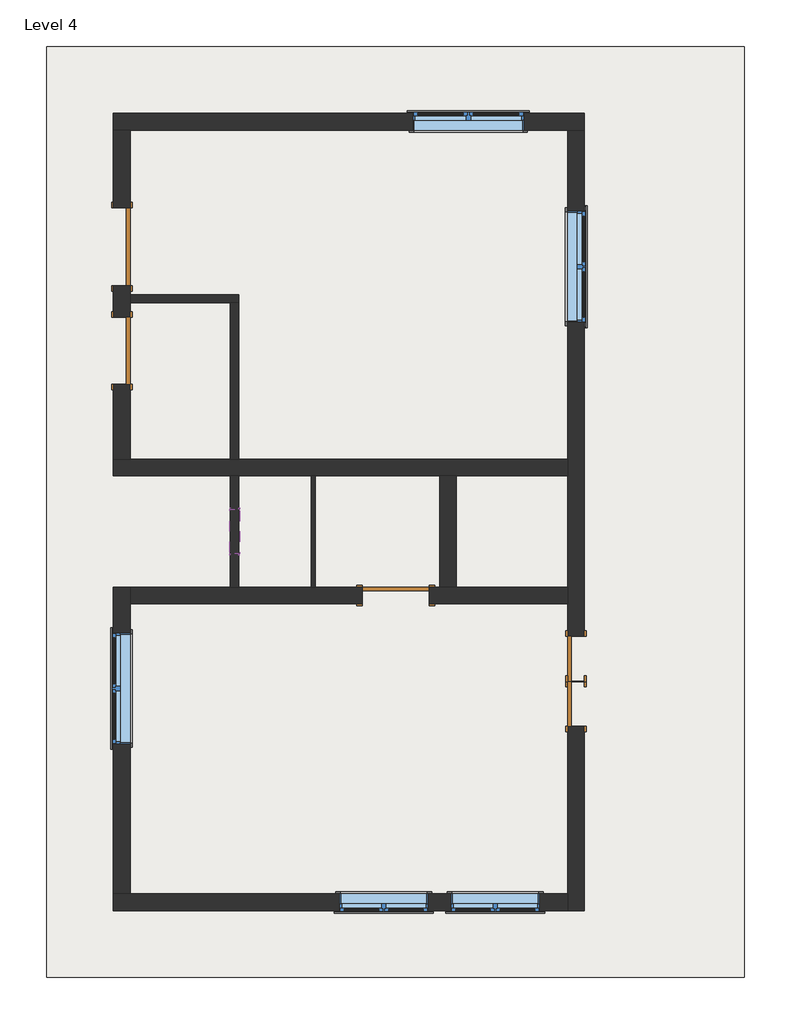
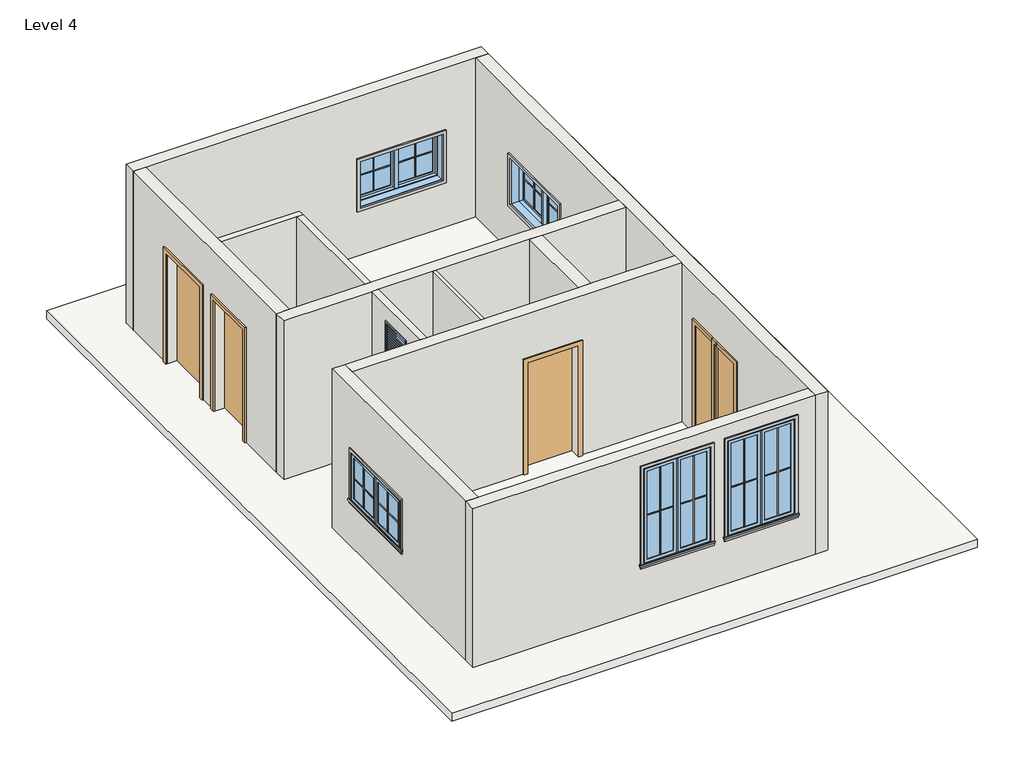
# One storey, incomplete: 20 proxies, 12 walls, 6 windows, 5 doors, 1 roof.
"""IFC4 building model written with IfcOpenShell, lengths in millimetres."""

from ifc_helpers import new_model, si_unit, frame, origin, place, context, project, spatial, polyline, outline, extrude, faceted_brep, transform, mapped, element, save
from components import muntin_pattern_2x2_muntin_pattern_2x2_9352d081, muntin_pattern_2x2_muntin_pattern_2x2_5c2cbe28, muntin_pattern_2x2_muntin_pattern_2x2_2b4d9f72, muntin_pattern_2x2_muntin_pattern_2x2_ef995ed3, trim_window_exterior_flat_with_sill_979bde60, trim_window_exterior_flat_with_sill_b7e4d11c, trim_window_interior_flat_picture_frame_7883d11b, trim_window_interior_flat_picture_frame_936b8d2a, single_flush_door_2_0d3b4037, single_flush_door_2_4a3212df, door_a90ba1ad, door_0ca8825f, door_9d399b00, window_casement_double_c1d95f0f, window_casement_double_wall_4_6ca1769e, window_d39e7ecb

model = new_model("IFC4")

# Units and contexts
model_context = context("Model", 3, world=origin())
ifc_project = project(units=[si_unit("LENGTHUNIT", "METRE", prefix="MILLI")], contexts=[model_context])

# Site, building, storey
site = spatial("IfcSite", under=ifc_project)
building = spatial("IfcBuilding", under=site)
storey = spatial("IfcBuildingStorey", under=building, Name="Level 4", Elevation=6400.8)

# Proxies
placement = place(None, origin())
muntin_pattern_2x2_muntin_pattern_2x2_shape = muntin_pattern_2x2_muntin_pattern_2x2_9352d081(model_context)
element("IfcBuildingElementProxy", 1, Name="Muntin Pattern_2x2 : Muntin Pattern_2x2", ObjectType="Muntin Pattern_2x2 : Muntin Pattern_2x2", at=placement, inside=storey, context=model_context, shape_type="MappedRepresentation", body=[
    mapped(muntin_pattern_2x2_muntin_pattern_2x2_shape, transform((-4785.3510342, -2707.8617544, 7385.05), x_axis=(0.0, 1.0, 0.0), y_axis=(-1.0, 0.0, 0.0), z_axis=(0.0, 0.0, 1.0))),
])
element("IfcBuildingElementProxy", 2, Name="Muntin Pattern_2x2 : Muntin Pattern_2x2", ObjectType="Muntin Pattern_2x2 : Muntin Pattern_2x2", at=placement, inside=storey, context=model_context, shape_type="MappedRepresentation", body=[
    mapped(muntin_pattern_2x2_muntin_pattern_2x2_shape, transform((1634.4989658, 3816.7632456, 7385.05), x_axis=(0.0, -1.0, 0.0), y_axis=(1.0, 0.0, 0.0), z_axis=(0.0, 0.0, 1.0))),
])
element("IfcBuildingElementProxy", 3, Name="Muntin Pattern_2x2 : Muntin Pattern_2x2", ObjectType="Muntin Pattern_2x2 : Muntin Pattern_2x2", at=placement, inside=storey, context=model_context, shape_type="MappedRepresentation", body=[
    mapped(muntin_pattern_2x2_muntin_pattern_2x2_shape, transform((-322.8885342, 5523.3257456, 7385.05), x_axis=(1.0, 0.0, 0.0), y_axis=(0.0, 1.0, 0.0), z_axis=(0.0, 0.0, 1.0))),
])
muntin_pattern_2x2_muntin_pattern_2x2_2_shape = muntin_pattern_2x2_muntin_pattern_2x2_5c2cbe28(model_context)
element("IfcBuildingElementProxy", 4, Name="Muntin Pattern_2x2 : Muntin Pattern_2x2", ObjectType="Muntin Pattern_2x2 : Muntin Pattern_2x2", at=placement, inside=storey, context=model_context, shape_type="MappedRepresentation", body=[
    mapped(muntin_pattern_2x2_muntin_pattern_2x2_2_shape, transform((-4785.3510342, -1949.0367544, 7385.05), x_axis=(0.0, -1.0, 0.0), y_axis=(1.0, 0.0, 0.0), z_axis=(0.0, 0.0, 1.0))),
])
element("IfcBuildingElementProxy", 5, Name="Muntin Pattern_2x2 : Muntin Pattern_2x2", ObjectType="Muntin Pattern_2x2 : Muntin Pattern_2x2", at=placement, inside=storey, context=model_context, shape_type="MappedRepresentation", body=[
    mapped(muntin_pattern_2x2_muntin_pattern_2x2_2_shape, transform((1634.4989658, 3057.9382456, 7385.05), x_axis=(0.0, 1.0, 0.0), y_axis=(-1.0, 0.0, 0.0), z_axis=(0.0, 0.0, 1.0))),
])
element("IfcBuildingElementProxy", 6, Name="Muntin Pattern_2x2 : Muntin Pattern_2x2", ObjectType="Muntin Pattern_2x2 : Muntin Pattern_2x2", at=placement, inside=storey, context=model_context, shape_type="MappedRepresentation", body=[
    mapped(muntin_pattern_2x2_muntin_pattern_2x2_2_shape, transform((435.9364658, 5523.3257456, 7385.05), x_axis=(-1.0, 0.0, 0.0), y_axis=(0.0, -1.0, 0.0), z_axis=(0.0, 0.0, 1.0))),
])
muntin_pattern_2x2_muntin_pattern_2x2_3_shape = muntin_pattern_2x2_muntin_pattern_2x2_2b4d9f72(model_context)
element("IfcBuildingElementProxy", 7, Name="Muntin Pattern_2x2 : Muntin Pattern_2x2", ObjectType="Muntin Pattern_2x2 : Muntin Pattern_2x2", at=placement, inside=storey, context=model_context, shape_type="MappedRepresentation", body=[
    mapped(muntin_pattern_2x2_muntin_pattern_2x2_3_shape, transform((-795.9635342, -5354.2242544, 7385.05), x_axis=(-1.0, 0.0, 0.0), y_axis=(0.0, -1.0, 0.0), z_axis=(0.0, 0.0, 1.0))),
])
element("IfcBuildingElementProxy", 8, Name="Muntin Pattern_2x2 : Muntin Pattern_2x2", ObjectType="Muntin Pattern_2x2 : Muntin Pattern_2x2", at=placement, inside=storey, context=model_context, shape_type="MappedRepresentation", body=[
    mapped(muntin_pattern_2x2_muntin_pattern_2x2_3_shape, transform((728.0364658, -5354.2242544, 7385.05), x_axis=(-1.0, 0.0, 0.0), y_axis=(0.0, -1.0, 0.0), z_axis=(0.0, 0.0, 1.0))),
])
muntin_pattern_2x2_muntin_pattern_2x2_4_shape = muntin_pattern_2x2_muntin_pattern_2x2_ef995ed3(model_context)
element("IfcBuildingElementProxy", 9, Name="Muntin Pattern_2x2 : Muntin Pattern_2x2", ObjectType="Muntin Pattern_2x2 : Muntin Pattern_2x2", at=placement, inside=storey, context=model_context, shape_type="MappedRepresentation", body=[
    mapped(muntin_pattern_2x2_muntin_pattern_2x2_4_shape, transform((-1402.3885342, -5354.2242544, 7385.05), x_axis=(1.0, 0.0, 0.0), y_axis=(0.0, 1.0, 0.0), z_axis=(0.0, 0.0, 1.0))),
])
element("IfcBuildingElementProxy", 10, Name="Muntin Pattern_2x2 : Muntin Pattern_2x2", ObjectType="Muntin Pattern_2x2 : Muntin Pattern_2x2", at=placement, inside=storey, context=model_context, shape_type="MappedRepresentation", body=[
    mapped(muntin_pattern_2x2_muntin_pattern_2x2_4_shape, transform((121.6114658, -5354.2242544, 7385.05), x_axis=(1.0, 0.0, 0.0), y_axis=(0.0, 1.0, 0.0), z_axis=(0.0, 0.0, 1.0))),
])
trim_window_exterior_flat_with_sill_shape = trim_window_exterior_flat_with_sill_979bde60(model_context)
element("IfcBuildingElementProxy", 11, Name="Trim-Window-Exterior-Flat : with Sill", ObjectType="Trim-Window-Exterior-Flat : with Sill", at=placement, inside=storey, context=model_context, shape_type="MappedRepresentation", body=[
    mapped(trim_window_exterior_flat_with_sill_shape, transform((-4794.8760342, -2328.4492544, 8229.6), x_axis=(0.0, -1.0, 0.0), y_axis=(0.0, 0.0, 1.0), z_axis=(-1.0, 0.0, 0.0))),
])
element("IfcBuildingElementProxy", 12, Name="Trim-Window-Exterior-Flat : with Sill", ObjectType="Trim-Window-Exterior-Flat : with Sill", at=placement, inside=storey, context=model_context, shape_type="MappedRepresentation", body=[
    mapped(trim_window_exterior_flat_with_sill_shape, transform((1644.0239658, 3437.3507456, 8229.6), x_axis=(0.0, 1.0, 0.0), y_axis=(0.0, 0.0, 1.0), z_axis=(1.0, 0.0, 0.0))),
])
element("IfcBuildingElementProxy", 13, Name="Trim-Window-Exterior-Flat : with Sill", ObjectType="Trim-Window-Exterior-Flat : with Sill", at=placement, inside=storey, context=model_context, shape_type="MappedRepresentation", body=[
    mapped(trim_window_exterior_flat_with_sill_shape, transform((56.5239658, 5532.8507456, 8229.6), x_axis=(-1.0, 0.0, 0.0), y_axis=(0.0, 0.0, 1.0), z_axis=(0.0, 1.0, 0.0))),
])
trim_window_exterior_flat_with_sill_2_shape = trim_window_exterior_flat_with_sill_b7e4d11c(model_context)
element("IfcBuildingElementProxy", 14, Name="Trim-Window-Exterior-Flat : with Sill", ObjectType="Trim-Window-Exterior-Flat : with Sill", at=placement, inside=storey, context=model_context, shape_type="MappedRepresentation", body=[
    mapped(trim_window_exterior_flat_with_sill_2_shape, transform((-1099.1760342, -5363.7492544, 9144.0), x_axis=(1.0, 0.0, 0.0), y_axis=(0.0, 0.0, 1.0), z_axis=(0.0, -1.0, 0.0))),
])
element("IfcBuildingElementProxy", 15, Name="Trim-Window-Exterior-Flat : with Sill", ObjectType="Trim-Window-Exterior-Flat : with Sill", at=placement, inside=storey, context=model_context, shape_type="MappedRepresentation", body=[
    mapped(trim_window_exterior_flat_with_sill_2_shape, transform((424.8239658, -5363.7492544, 9144.0), x_axis=(1.0, 0.0, 0.0), y_axis=(0.0, 0.0, 1.0), z_axis=(0.0, -1.0, 0.0))),
])
trim_window_interior_flat_picture_frame_shape = trim_window_interior_flat_picture_frame_7883d11b(model_context)
element("IfcBuildingElementProxy", 16, Name="Trim-Window-Interior-Flat : Picture Frame", ObjectType="Trim-Window-Interior-Flat : Picture Frame", at=placement, inside=storey, context=model_context, shape_type="MappedRepresentation", body=[
    mapped(trim_window_interior_flat_picture_frame_shape, transform((-4566.2760342, -2328.4492544, 8229.6), x_axis=(0.0, 1.0, 0.0), y_axis=(0.0, 0.0, 1.0), z_axis=(1.0, 0.0, 0.0))),
])
element("IfcBuildingElementProxy", 17, Name="Trim-Window-Interior-Flat : Picture Frame", ObjectType="Trim-Window-Interior-Flat : Picture Frame", at=placement, inside=storey, context=model_context, shape_type="MappedRepresentation", body=[
    mapped(trim_window_interior_flat_picture_frame_shape, transform((1415.4239658, 3437.3507456, 8229.6), x_axis=(0.0, -1.0, 0.0), y_axis=(0.0, 0.0, 1.0), z_axis=(-1.0, 0.0, 0.0))),
])
element("IfcBuildingElementProxy", 18, Name="Trim-Window-Interior-Flat : Picture Frame", ObjectType="Trim-Window-Interior-Flat : Picture Frame", at=placement, inside=storey, context=model_context, shape_type="MappedRepresentation", body=[
    mapped(trim_window_interior_flat_picture_frame_shape, transform((56.5239658, 5304.2507456, 8229.6), x_axis=(1.0, 0.0, 0.0), y_axis=(0.0, 0.0, 1.0), z_axis=(0.0, -1.0, 0.0))),
])
trim_window_interior_flat_picture_frame_2_shape = trim_window_interior_flat_picture_frame_936b8d2a(model_context)
element("IfcBuildingElementProxy", 19, Name="Trim-Window-Interior-Flat : Picture Frame", ObjectType="Trim-Window-Interior-Flat : Picture Frame", at=placement, inside=storey, context=model_context, shape_type="MappedRepresentation", body=[
    mapped(trim_window_interior_flat_picture_frame_2_shape, transform((-1099.1760342, -5135.1492544, 9144.0), x_axis=(-1.0, 0.0, 0.0), y_axis=(0.0, 0.0, 1.0), z_axis=(0.0, 1.0, 0.0))),
])
element("IfcBuildingElementProxy", 20, Name="Trim-Window-Interior-Flat : Picture Frame", ObjectType="Trim-Window-Interior-Flat : Picture Frame", at=placement, inside=storey, context=model_context, shape_type="MappedRepresentation", body=[
    mapped(trim_window_interior_flat_picture_frame_2_shape, transform((424.8239658, -5135.1492544, 9144.0), x_axis=(-1.0, 0.0, 0.0), y_axis=(0.0, 0.0, 1.0), z_axis=(0.0, 1.0, 0.0))),
])

# Doors
single_flush_door_2_shape = single_flush_door_2_0d3b4037(model_context)
element("IfcDoor", 21, ObjectType="Single-Flush : door 2'", at=placement, inside=storey, context=model_context, shape_type="MappedRepresentation", body=[
    mapped(single_flush_door_2_shape, transform((1529.7239658, -1922.0492544, 6400.8), x_axis=(0.0, 1.0, 0.0), y_axis=(-1.0, 0.0, 0.0), z_axis=(0.0, 0.0, 1.0))),
])
single_flush_door_2_2_shape = single_flush_door_2_4a3212df(model_context)
element("IfcDoor", 22, ObjectType="Single-Flush : door 2'", at=placement, inside=storey, context=model_context, shape_type="MappedRepresentation", body=[
    mapped(single_flush_door_2_2_shape, transform((1529.7239658, -2537.9992544, 6400.8), x_axis=(0.0, -1.0, 0.0), y_axis=(1.0, 0.0, 0.0), z_axis=(0.0, 0.0, 1.0))),
])
door_shape = door_a90ba1ad(model_context)
element("IfcDoor", 23, ObjectType="Single-Flush : door 2'6\"", at=placement, inside=storey, context=model_context, shape_type="MappedRepresentation", body=[
    mapped(door_shape, transform((-4680.5760342, 2288.0007456, 6400.8), x_axis=(0.0, 1.0, 0.0), y_axis=(-1.0, 0.0, 0.0), z_axis=(0.0, 0.0, 1.0))),
])
door_2_shape = door_0ca8825f(model_context)
element("IfcDoor", 24, ObjectType="Single-Flush : door 2'6\"", at=placement, inside=storey, context=model_context, shape_type="MappedRepresentation", body=[
    mapped(door_2_shape, transform((-934.0760342, -1058.4492544, 6400.8), x_axis=(1.0, 0.0, 0.0), y_axis=(0.0, 1.0, 0.0), z_axis=(0.0, 0.0, 1.0))),
])
door_3_shape = door_9d399b00(model_context)
element("IfcDoor", 25, ObjectType="Single-Flush : door 3'6\"", at=placement, inside=storey, context=model_context, shape_type="MappedRepresentation", body=[
    mapped(door_3_shape, transform((-4680.5760342, 3710.4007456, 6400.8), x_axis=(0.0, -1.0, 0.0), y_axis=(1.0, 0.0, 0.0), z_axis=(0.0, 0.0, 1.0))),
])

# Roof
element("IfcRoof", 26, ObjectType="roof 6\"", at=placement, inside=storey, context=model_context, shape_type="SweptSolid", body=[
    extrude(outline(polyline([(-5709.2760342, 6447.2507456), (3828.4239658, 6447.2507456), (3828.4239658, -6278.1492544), (-5709.2760342, -6278.1492544), (-5709.2760342, 6447.2507456)])), frame((0.0, 0.0, 6248.4), z_axis=(0.0, 0.0, 1.0), x_axis=(1.0, 0.0, 0.0)), (0.0, 0.0, 1.0), 152.4),
])

# Walls
element("IfcWall", 27, ObjectType="wall 2\"", at=placement, inside=storey, context=model_context, shape_type="SweptSolid", body=[
    extrude(outline(polyline([(-2089.7760342, -944.1492544), (-2089.7760342, 579.8507456), (-2038.9760342, 579.8507456), (-2038.9760342, -944.1492544), (-2089.7760342, -944.1492544)])), frame((0.0, 0.0, 6400.8), z_axis=(0.0, 0.0, 1.0), x_axis=(1.0, 0.0, 0.0)), (0.0, 0.0, 1.0), 3048.0),
])
element("IfcWall", 28, ObjectType="wall 4.5\"", at=placement, inside=storey, context=model_context, shape_type="Brep", body=[
    faceted_brep([(-4566.2760342, 2942.0507456, 6400.8), (-3194.6760342, 2942.0507456, 6400.8), (-3080.3760342, 2942.0507456, 6400.8), (-3080.3760342, 2942.0507456, 9448.8), (-3194.6760342, 2942.0507456, 9448.8), (-4566.2760342, 2942.0507456, 9448.8), (-4566.2760342, 3056.3507456, 6400.8), (-4566.2760342, 3056.3507456, 9448.8), (-3080.3760342, 3056.3507456, 9448.8), (-3080.3760342, 3056.3507456, 6400.8)], [[[0, 1, 2, 3, 4, 5]], [[6, 7, 8, 9]], [[2, 1, 0, 6, 9]], [[0, 5, 7, 6]], [[3, 2, 9, 8]], [[5, 4, 3, 8, 7]]]),
])
element("IfcWall", 29, ObjectType="wall 4.5\"", at=placement, inside=storey, context=model_context, shape_type="SweptSolid", body=[
    extrude(outline(polyline([(-3194.6760342, 808.4507456), (-3194.6760342, 2942.0507456), (-3080.3760342, 2942.0507456), (-3080.3760342, 808.4507456), (-3194.6760342, 808.4507456)])), frame((0.0, 0.0, 6400.8), z_axis=(0.0, 0.0, 1.0), x_axis=(1.0, 0.0, 0.0)), (0.0, 0.0, 1.0), 3048.0),
])
element("IfcWall", 30, ObjectType="wall 4.5\"", at=placement, inside=storey, context=model_context, shape_type="SweptSolid", body=[
    extrude(outline(polyline([(579.8507456, 6400.8), (-944.1492544, 6400.8), (-944.1492544, 9448.8), (579.8507456, 9448.8), (579.8507456, 6400.8)]), holes=[polyline([(-486.9492544, 9144.0), (-486.9492544, 8534.4), (122.6507456, 8534.4), (122.6507456, 9144.0), (-486.9492544, 9144.0)])]), frame((-3194.6760342, 0.0, 0.0), z_axis=(1.0, 0.0, 0.0), x_axis=(0.0, 1.0, 0.0)), (0.0, 0.0, 1.0), 114.3),
])
element("IfcWall", 31, ObjectType="wall 9\"", at=placement, inside=storey, context=model_context, shape_type="Brep", body=[
    faceted_brep([(-4794.8760342, 5304.2507456, 6400.8), (-4566.2760342, 5304.2507456, 6400.8), (1415.4239658, 5304.2507456, 6400.8), (1644.0239658, 5304.2507456, 6400.8), (1644.0239658, 5304.2507456, 9448.8), (1415.4239658, 5304.2507456, 9448.8), (-4566.2760342, 5304.2507456, 9448.8), (-4794.8760342, 5304.2507456, 9448.8), (818.5239658, 5304.2507456, 8229.6), (818.5239658, 5304.2507456, 7315.2), (-705.4760342, 5304.2507456, 7315.2), (-705.4760342, 5304.2507456, 8229.6), (-4794.8760342, 5532.8507456, 6400.8), (-4794.8760342, 5532.8507456, 9448.8), (1644.0239658, 5532.8507456, 9448.8), (1644.0239658, 5532.8507456, 6400.8), (818.5239658, 5532.8507456, 8229.6), (-705.4760342, 5532.8507456, 8229.6), (-705.4760342, 5532.8507456, 7315.2), (818.5239658, 5532.8507456, 7315.2)], [[[0, 1, 2, 3, 4, 5, 6, 7], [8, 9, 10, 11]], [[12, 13, 14, 15], [16, 17, 18, 19]], [[3, 2, 1, 0, 12, 15]], [[4, 3, 15, 14]], [[0, 7, 13, 12]], [[9, 8, 16, 19]], [[10, 9, 19, 18]], [[11, 10, 18, 17]], [[8, 11, 17, 16]], [[7, 6, 5, 4, 14, 13]]]),
])
element("IfcWall", 32, ObjectType="wall 9\"", at=placement, inside=storey, context=model_context, shape_type="Brep", body=[
    faceted_brep([(1415.4239658, 5304.2507456, 9448.8), (1415.4239658, 5304.2507456, 6400.8), (1415.4239658, 808.4507456, 6400.8), (1415.4239658, 579.8507456, 6400.8), (1415.4239658, -944.1492544, 6400.8), (1415.4239658, -1172.7492544, 6400.8), (1415.4239658, -1617.2492544, 6400.8), (1415.4239658, -1617.2492544, 8534.4), (1415.4239658, -2226.8492544, 8534.4), (1415.4239658, -2226.8492544, 6400.8), (1415.4239658, -2233.1992544, 6400.8), (1415.4239658, -2233.1992544, 8534.4), (1415.4239658, -2842.7992544, 8534.4), (1415.4239658, -2842.7992544, 6400.8), (1415.4239658, -5135.1492544, 6400.8), (1415.4239658, -5363.7492544, 6400.8), (1415.4239658, -5363.7492544, 9448.8), (1415.4239658, -5135.1492544, 9448.8), (1415.4239658, -1172.7492544, 9448.8), (1415.4239658, -944.1492544, 9448.8), (1415.4239658, 579.8507456, 9448.8), (1415.4239658, 808.4507456, 9448.8), (1415.4239658, 2675.3507456, 8229.6), (1415.4239658, 2675.3507456, 7315.2), (1415.4239658, 4199.3507456, 7315.2), (1415.4239658, 4199.3507456, 8229.6), (1644.0239658, 5304.2507456, 6400.8), (1644.0239658, 5304.2507456, 9448.8), (1644.0239658, -5363.7492544, 9448.8), (1644.0239658, -5363.7492544, 6400.8), (1644.0239658, -2842.7992544, 6400.8), (1644.0239658, -2842.7992544, 8534.4), (1644.0239658, -2233.1992544, 8534.4), (1644.0239658, -2233.1992544, 6400.8), (1644.0239658, -2226.8492544, 6400.8), (1644.0239658, -2226.8492544, 8534.4), (1644.0239658, -1617.2492544, 8534.4), (1644.0239658, -1617.2492544, 6400.8), (1644.0239658, 2675.3507456, 8229.6), (1644.0239658, 4199.3507456, 8229.6), (1644.0239658, 4199.3507456, 7315.2), (1644.0239658, 2675.3507456, 7315.2)], [[[0, 1, 2, 3, 4, 5, 6, 7, 8, 9, 10, 11, 12, 13, 14, 15, 16, 17, 18, 19, 20, 21], [22, 23, 24, 25]], [[26, 27, 28, 29, 30, 31, 32, 33, 34, 35, 36, 37], [38, 39, 40, 41]], [[1, 26, 37, 6, 5, 4, 3, 2]], [[29, 15, 14, 13, 30]], [[9, 34, 33, 10]], [[1, 0, 27, 26]], [[16, 15, 29, 28]], [[23, 22, 38, 41]], [[24, 23, 41, 40]], [[25, 24, 40, 39]], [[22, 25, 39, 38]], [[7, 6, 37, 36]], [[8, 7, 36, 35]], [[9, 8, 35, 34]], [[12, 31, 30, 13]], [[31, 12, 11, 32]], [[32, 11, 10, 33]], [[0, 21, 20, 19, 18, 17, 16, 28, 27]]]),
])
element("IfcWall", 33, ObjectType="wall 9\"", at=placement, inside=storey, context=model_context, shape_type="Brep", body=[
    faceted_brep([(1415.4239658, 808.4507456, 6400.8), (-3080.3760342, 808.4507456, 6400.8), (-3194.6760342, 808.4507456, 6400.8), (-4566.2760342, 808.4507456, 6400.8), (-4794.8760342, 808.4507456, 6400.8), (-4794.8760342, 808.4507456, 9448.8), (-4566.2760342, 808.4507456, 9448.8), (-3194.6760342, 808.4507456, 9448.8), (-3080.3760342, 808.4507456, 9448.8), (1415.4239658, 808.4507456, 9448.8), (1415.4239658, 579.8507456, 6400.8), (1415.4239658, 579.8507456, 9448.8), (-108.5760342, 579.8507456, 9448.8), (-337.1760342, 579.8507456, 9448.8), (-2038.9760342, 579.8507456, 9448.8), (-2089.7760342, 579.8507456, 9448.8), (-3080.3760342, 579.8507456, 9448.8), (-3194.6760342, 579.8507456, 9448.8), (-4794.8760342, 579.8507456, 9448.8), (-4794.8760342, 579.8507456, 6400.8), (-3194.6760342, 579.8507456, 6400.8), (-3080.3760342, 579.8507456, 6400.8), (-2089.7760342, 579.8507456, 6400.8), (-2038.9760342, 579.8507456, 6400.8), (-337.1760342, 579.8507456, 6400.8), (-108.5760342, 579.8507456, 6400.8)], [[[0, 1, 2, 3, 4, 5, 6, 7, 8, 9]], [[10, 11, 12, 13, 14, 15, 16, 17, 18, 19, 20, 21, 22, 23, 24, 25]], [[4, 3, 2, 1, 0, 10, 25, 24, 23, 22, 21, 20, 19]], [[0, 9, 11, 10]], [[5, 4, 19, 18]], [[9, 8, 7, 6, 5, 18, 17, 16, 15, 14, 13, 12, 11]]]),
])
element("IfcWall", 34, ObjectType="wall 9\"", at=placement, inside=storey, context=model_context, shape_type="Brep", body=[
    faceted_brep([(-4566.2760342, 2745.2007456, 8534.4), (-4566.2760342, 2745.2007456, 6400.8), (-4566.2760342, 2942.0507456, 6400.8), (-4566.2760342, 3056.3507456, 6400.8), (-4566.2760342, 3177.0007456, 6400.8), (-4566.2760342, 3177.0007456, 8534.4), (-4566.2760342, 4243.8007456, 8534.4), (-4566.2760342, 4243.8007456, 6400.8), (-4566.2760342, 5304.2507456, 6400.8), (-4566.2760342, 5304.2507456, 9448.8), (-4566.2760342, 3056.3507456, 9448.8), (-4566.2760342, 2942.0507456, 9448.8), (-4566.2760342, 808.4507456, 9448.8), (-4566.2760342, 808.4507456, 6400.8), (-4566.2760342, 1830.8007456, 6400.8), (-4566.2760342, 1830.8007456, 8534.4), (-4794.8760342, 3177.0007456, 6400.8), (-4794.8760342, 2745.2007456, 6400.8), (-4794.8760342, 2745.2007456, 8534.4), (-4794.8760342, 1830.8007456, 8534.4), (-4794.8760342, 1830.8007456, 6400.8), (-4794.8760342, 808.4507456, 6400.8), (-4794.8760342, 808.4507456, 9448.8), (-4794.8760342, 5304.2507456, 9448.8), (-4794.8760342, 5304.2507456, 6400.8), (-4794.8760342, 4243.8007456, 6400.8), (-4794.8760342, 4243.8007456, 8534.4), (-4794.8760342, 3177.0007456, 8534.4)], [[[0, 1, 2, 3, 4, 5, 6, 7, 8, 9, 10, 11, 12, 13, 14, 15]], [[16, 17, 18, 19, 20, 21, 22, 23, 24, 25, 26, 27]], [[25, 24, 8, 7]], [[14, 13, 21, 20]], [[4, 3, 2, 1, 17, 16]], [[9, 8, 24, 23]], [[13, 12, 22, 21]], [[5, 4, 16, 27]], [[6, 5, 27, 26]], [[7, 6, 26, 25]], [[18, 17, 1, 0]], [[19, 18, 0, 15]], [[20, 19, 15, 14]], [[12, 11, 10, 9, 23, 22]]]),
])
element("IfcWall", 35, ObjectType="wall 9\"", at=placement, inside=storey, context=model_context, shape_type="Brep", body=[
    faceted_brep([(1415.4239658, -5135.1492544, 6400.8), (-4566.2760342, -5135.1492544, 6400.8), (-4794.8760342, -5135.1492544, 6400.8), (-4794.8760342, -5135.1492544, 9448.8), (-4566.2760342, -5135.1492544, 9448.8), (1415.4239658, -5135.1492544, 9448.8), (-1708.7760342, -5135.1492544, 9144.0), (-1708.7760342, -5135.1492544, 7315.2), (-489.5760342, -5135.1492544, 7315.2), (-489.5760342, -5135.1492544, 9144.0), (-184.7760342, -5135.1492544, 9144.0), (-184.7760342, -5135.1492544, 7315.2), (1034.4239658, -5135.1492544, 7315.2), (1034.4239658, -5135.1492544, 9144.0), (1415.4239658, -5363.7492544, 6400.8), (1415.4239658, -5363.7492544, 9448.8), (-4794.8760342, -5363.7492544, 9448.8), (-4794.8760342, -5363.7492544, 6400.8), (-1708.7760342, -5363.7492544, 9144.0), (-489.5760342, -5363.7492544, 9144.0), (-489.5760342, -5363.7492544, 7315.2), (-1708.7760342, -5363.7492544, 7315.2), (-184.7760342, -5363.7492544, 9144.0), (1034.4239658, -5363.7492544, 9144.0), (1034.4239658, -5363.7492544, 7315.2), (-184.7760342, -5363.7492544, 7315.2)], [[[0, 1, 2, 3, 4, 5], [6, 7, 8, 9], [10, 11, 12, 13]], [[14, 15, 16, 17], [18, 19, 20, 21], [22, 23, 24, 25]], [[2, 1, 0, 14, 17]], [[0, 5, 15, 14]], [[3, 2, 17, 16]], [[7, 6, 18, 21]], [[8, 7, 21, 20]], [[9, 8, 20, 19]], [[6, 9, 19, 18]], [[11, 10, 22, 25]], [[12, 11, 25, 24]], [[13, 12, 24, 23]], [[10, 13, 23, 22]], [[5, 4, 3, 16, 15]]]),
])
element("IfcWall", 36, ObjectType="wall 9\"", at=placement, inside=storey, context=model_context, shape_type="Brep", body=[
    faceted_brep([(-4566.2760342, -5135.1492544, 6400.8), (-4566.2760342, -1172.7492544, 6400.8), (-4566.2760342, -944.1492544, 6400.8), (-4566.2760342, -944.1492544, 9448.8), (-4566.2760342, -1172.7492544, 9448.8), (-4566.2760342, -5135.1492544, 9448.8), (-4566.2760342, -1566.4492544, 8229.6), (-4566.2760342, -1566.4492544, 7315.2), (-4566.2760342, -3090.4492544, 7315.2), (-4566.2760342, -3090.4492544, 8229.6), (-4794.8760342, -5135.1492544, 6400.8), (-4794.8760342, -5135.1492544, 9448.8), (-4794.8760342, -944.1492544, 9448.8), (-4794.8760342, -944.1492544, 6400.8), (-4794.8760342, -1566.4492544, 8229.6), (-4794.8760342, -3090.4492544, 8229.6), (-4794.8760342, -3090.4492544, 7315.2), (-4794.8760342, -1566.4492544, 7315.2)], [[[0, 1, 2, 3, 4, 5], [6, 7, 8, 9]], [[10, 11, 12, 13], [14, 15, 16, 17]], [[2, 1, 0, 10, 13]], [[0, 5, 11, 10]], [[3, 2, 13, 12]], [[7, 6, 14, 17]], [[8, 7, 17, 16]], [[9, 8, 16, 15]], [[6, 9, 15, 14]], [[5, 4, 3, 12, 11]]]),
])
element("IfcWall", 37, ObjectType="wall 9\"", at=placement, inside=storey, context=model_context, shape_type="Brep", body=[
    faceted_brep([(-476.8760342, -1172.7492544, 8534.4), (-476.8760342, -1172.7492544, 6400.8), (1415.4239658, -1172.7492544, 6400.8), (1415.4239658, -1172.7492544, 9448.8), (-4566.2760342, -1172.7492544, 9448.8), (-4566.2760342, -1172.7492544, 6400.8), (-1391.2760342, -1172.7492544, 6400.8), (-1391.2760342, -1172.7492544, 8534.4), (1415.4239658, -944.1492544, 6400.8), (-108.5760342, -944.1492544, 6400.8), (-337.1760342, -944.1492544, 6400.8), (-476.8760342, -944.1492544, 6400.8), (-476.8760342, -944.1492544, 8534.4), (-1391.2760342, -944.1492544, 8534.4), (-1391.2760342, -944.1492544, 6400.8), (-2038.9760342, -944.1492544, 6400.8), (-2089.7760342, -944.1492544, 6400.8), (-3080.3760342, -944.1492544, 6400.8), (-3194.6760342, -944.1492544, 6400.8), (-4566.2760342, -944.1492544, 6400.8), (-4566.2760342, -944.1492544, 9448.8), (-3194.6760342, -944.1492544, 9448.8), (-3080.3760342, -944.1492544, 9448.8), (-2089.7760342, -944.1492544, 9448.8), (-2038.9760342, -944.1492544, 9448.8), (-337.1760342, -944.1492544, 9448.8), (-108.5760342, -944.1492544, 9448.8), (1415.4239658, -944.1492544, 9448.8)], [[[0, 1, 2, 3, 4, 5, 6, 7]], [[8, 9, 10, 11, 12, 13, 14, 15, 16, 17, 18, 19, 20, 21, 22, 23, 24, 25, 26, 27]], [[6, 5, 19, 18, 17, 16, 15, 14]], [[2, 1, 11, 10, 9, 8]], [[5, 4, 20, 19]], [[3, 2, 8, 27]], [[12, 11, 1, 0]], [[13, 12, 0, 7]], [[14, 13, 7, 6]], [[4, 3, 27, 26, 25, 24, 23, 22, 21, 20]]]),
])
element("IfcWall", 38, ObjectType="wall 9\"", at=placement, inside=storey, context=model_context, shape_type="SweptSolid", body=[
    extrude(outline(polyline([(-108.5760342, 579.8507456), (-108.5760342, -944.1492544), (-337.1760342, -944.1492544), (-337.1760342, 579.8507456), (-108.5760342, 579.8507456)])), frame((0.0, 0.0, 6400.8), z_axis=(0.0, 0.0, 1.0), x_axis=(1.0, 0.0, 0.0)), (0.0, 0.0, 1.0), 3048.0),
])

# Windows
window_casement_double_shape = window_casement_double_c1d95f0f(model_context)
element("IfcWindow", 39, ObjectType="Window-Casement-Double", at=placement, inside=storey, context=model_context, shape_type="MappedRepresentation", body=[
    mapped(window_casement_double_shape, transform((-4680.5760342, -2328.4492544, 6400.8), x_axis=(0.0, 1.0, 0.0), y_axis=(-1.0, 0.0, 0.0), z_axis=(0.0, 0.0, 1.0))),
])
element("IfcWindow", 40, ObjectType="Window-Casement-Double", at=placement, inside=storey, context=model_context, shape_type="MappedRepresentation", body=[
    mapped(window_casement_double_shape, transform((1529.7239658, 3437.3507456, 6400.8), x_axis=(0.0, -1.0, 0.0), y_axis=(1.0, 0.0, 0.0), z_axis=(0.0, 0.0, 1.0))),
])
element("IfcWindow", 41, ObjectType="Window-Casement-Double", at=placement, inside=storey, context=model_context, shape_type="MappedRepresentation", body=[
    mapped(window_casement_double_shape, transform((56.5239658, 5418.5507456, 6400.8), x_axis=(1.0, 0.0, 0.0), y_axis=(0.0, 1.0, 0.0), z_axis=(0.0, 0.0, 1.0))),
])
window_casement_double_wall_4_shape = window_casement_double_wall_4_6ca1769e(model_context)
element("IfcWindow", 42, ObjectType="Window-Casement-Double : wall 4'", at=placement, inside=storey, context=model_context, shape_type="MappedRepresentation", body=[
    mapped(window_casement_double_wall_4_shape, transform((-1099.1760342, -5249.4492544, 6400.8), x_axis=(-1.0, 0.0, 0.0), y_axis=(0.0, -1.0, 0.0), z_axis=(0.0, 0.0, 1.0))),
])
element("IfcWindow", 43, ObjectType="Window-Casement-Double : wall 4'", at=placement, inside=storey, context=model_context, shape_type="MappedRepresentation", body=[
    mapped(window_casement_double_wall_4_shape, transform((424.8239658, -5249.4492544, 6400.8), x_axis=(-1.0, 0.0, 0.0), y_axis=(0.0, -1.0, 0.0), z_axis=(0.0, 0.0, 1.0))),
])
window_shape = window_d39e7ecb(model_context)
element("IfcWindow", 44, ObjectType="Window-Louvers : 24\" x 24\"", at=placement, inside=storey, context=model_context, shape_type="MappedRepresentation", body=[
    mapped(window_shape, transform((-3143.8760342, -182.1492544, 7620.0), x_axis=(0.0, 1.0, 0.0), y_axis=(-1.0, 0.0, 0.0), z_axis=(0.0, 0.0, 1.0))),
])

save(model, "model.ifc")

# Revit data of these elements
# Type "Muntin Pattern_2x2 : Muntin Pattern_2x2"
#   Width [instance default] = 4' - 0"
#   Thickness = 0' - 0 1/2"
#   Height [instance default] = 4' - 0"
#   Distance = 0' - 0 3/4"
#   Interior Material [instance default] = none
#   Exterior Material [instance default] = none
#   Default Elevation = 0
# Type "Trim-Window-Exterior-Flat : with Sill"
#   Trim Width = 0' - 2 1/4"
#   Trim Thickness_Picture Frame = 0' - 1 1/4"
#   Trim Thickness_with Sill = 0' - 0 3/4"
#   Sill Thickness = 0' - 1 1/4"
#   Opening Width [instance default] = 2' - 0"
#   Opening Height [instance default] = 3' - 0"
#   Default Elevation = 4' - 0"
#   Sill = yes
#   Picture Frame = no
#   Trim Material [instance default] = none
# Type "Trim-Window-Interior-Flat : Picture Frame"
#   Trim Thickness_Picture Frame = 0' - 1 1/4"
#   Trim Width = 0' - 2 1/4"
#   Trim Thickness_with Sill = 0' - 0 3/4"
#   Sill Thickness = 0' - 1 1/4"
#   Opening Width [instance default] = 2' - 0"
#   Opening Height [instance default] = 3' - 0"
#   Default Elevation = 4' - 0"
#   Sill = no
#   Picture Frame = yes
#   Trim Material [instance default] = none
# Type "Single-Flush : door 2'"
#   Type Mark = "11"
#   Construction Type Id = "MDOOR"
#   Assembly Code = "C1020"
#   Analytic Construction = "Metal"
#   Thickness = 0' - 2"
#   Heat Transfer Coefficient (U) = 0.651978 BTU/(h·ft²·°F)
#   Height = 7' - 0"
#   Trim Projection Ext = 0' - 1"
#   Trim Projection Int = 0' - 1"
#   Trim Width = 0' - 3"
#   Width = 2' - 0"
#   Define Thermal Properties by = 1
#   Door Material = Door - Panel
#   Frame Material = Door - Frame
#   Visual Light Transmittance = 0
#   Solar Heat Gain Coefficient = 0
#   Function = (empty or 0)
#   Wall Closure = (empty or 0)
# Type "Single-Flush : door 2'6\""
#   Type Mark = "8"
#   Construction Type Id = "MDOOR"
#   Assembly Code = "C1020"
#   Analytic Construction = "Metal"
#   Thickness = 0' - 2"
#   Heat Transfer Coefficient (U) = 0.651978 BTU/(h·ft²·°F)
#   Height = 7' - 0"
#   Trim Projection Ext = 0' - 1"
#   Trim Projection Int = 0' - 1"
#   Trim Width = 0' - 3"
#   Width = 3' - 0"
#   Define Thermal Properties by = 1
#   Door Material = Door - Panel
#   Frame Material = Door - Frame
#   Visual Light Transmittance = 0
#   Solar Heat Gain Coefficient = 0
#   Function = (empty or 0)
#   Wall Closure = (empty or 0)
# Type "Single-Flush : door 3'6\""
#   Type Mark = "10"
#   Construction Type Id = "MDOOR"
#   Assembly Code = "C1020"
#   Analytic Construction = "Metal"
#   Thickness = 0' - 2"
#   Heat Transfer Coefficient (U) = 0.651978 BTU/(h·ft²·°F)
#   Height = 7' - 0"
#   Trim Projection Ext = 0' - 1"
#   Trim Projection Int = 0' - 1"
#   Trim Width = 0' - 3"
#   Width = 3' - 6"
#   Define Thermal Properties by = 1
#   Door Material = Door - Panel
#   Frame Material = Door - Frame
#   Visual Light Transmittance = 0
#   Solar Heat Gain Coefficient = 0
#   Function = (empty or 0)
#   Wall Closure = (empty or 0)
# Type "roof 6\""
#   Assembly Code = "B1020"
#   Layers, outside or top first: 0' - 6" no material (function 1)
# Type "wall 2\""
#   Assembly Code = "B2010"
#   Layers, outside or top first: 0' - 2" no material (function 1)
# Type "wall 4.5\""
#   Assembly Code = "B2010"
#   Layers, outside or top first: 0' - 4 1/2" no material (function 1)
# Type "wall 9\""
#   Assembly Code = "B2010"
#   Layers, outside or top first: 0' - 9" no material (function 1)
# Type "Window-Casement-Double"
#   Type Mark = "18"
#   Fire Rating = "0.5h"
#   Assembly Code = "B2020100"
#   Analytic Construction = "Double glazing - domestic"
#   Frame Extension [instance default] = 0' - 0 1/4"
#   Window Inset [instance default] = 0' - 0"
#   Wall Thickness [instance default] = 0' - 6"
#   Interior Wall Closure [instance default] = 0' - 2 1/4"
#   Half Width = 2' - 6"
#   Visual Light Transmittance = 0.81
#   Thermal Resistance (R) = 1.8146 (h·ft²·°F)/BTU
#   Solar Heat Gain Coefficient = 0.76
#   Rough Width = 5' - 0 1/2"
#   Rough Height = 3' - 0 1/2"
#   Height = 3' - 0"
#   Heat Transfer Coefficient (U) = 0.5511 BTU/(h·ft²·°F)
#   Exterior Wall Closure [instance default] = 0' - 1 1/4"
#   Extension Jamb [instance default] = 0' - 2 1/4"
#   Default Sill Height = 3' - 0"
#   Width = 5' - 0"
#   Muntin Visibility = yes
#   Interior Trim Visibility [instance default] = yes
#   Exterior Trim Visibility [instance default] = yes
#   Extension Jamb Visibility [instance default] = yes
#   Interior Trim Material = Wood - Stained
#   Muntin Pattern = Muntin Pattern_2x2 : Muntin Pattern_2x2
#   Interior Trim = Trim-Window-Interior-Flat : Picture Frame
#   Interior Frame Material = Wood - Stained
#   Glass Panel Material = Glass
#   Exterior Trim Material = Clad - White
#   Exterior Trim = Trim-Window-Exterior-Flat : with Sill
#   Exterior Frame Material = Clad - White
#   Wall Closure = (empty or 0)
# Type "Window-Casement-Double : wall 4'"
#   Type Mark = "19"
#   Fire Rating = "0.5h"
#   Assembly Code = "B2020100"
#   Analytic Construction = "Double glazing - domestic"
#   Frame Extension [instance default] = 0' - 0 1/4"
#   Window Inset [instance default] = 0' - 0"
#   Wall Thickness [instance default] = 0' - 6"
#   Interior Wall Closure [instance default] = 0' - 2 1/4"
#   Half Width = 2' - 0"
#   Visual Light Transmittance = 0.81
#   Thermal Resistance (R) = 1.8146 (h·ft²·°F)/BTU
#   Solar Heat Gain Coefficient = 0.76
#   Rough Width = 4' - 0 1/2"
#   Rough Height = 6' - 0 1/2"
#   Height = 6' - 0"
#   Heat Transfer Coefficient (U) = 0.5511 BTU/(h·ft²·°F)
#   Exterior Wall Closure [instance default] = 0' - 1 1/4"
#   Extension Jamb [instance default] = 0' - 2 1/4"
#   Default Sill Height = 3' - 0"
#   Width = 4' - 0"
#   Muntin Visibility = yes
#   Interior Trim Visibility [instance default] = yes
#   Exterior Trim Visibility [instance default] = yes
#   Extension Jamb Visibility [instance default] = yes
#   Interior Trim Material = Wood - Stained
#   Muntin Pattern = Muntin Pattern_2x2 : Muntin Pattern_2x2
#   Interior Trim = Trim-Window-Interior-Flat : Picture Frame
#   Interior Frame Material = Wood - Stained
#   Glass Panel Material = Glass
#   Exterior Trim Material = Clad - White
#   Exterior Trim = Trim-Window-Exterior-Flat : with Sill
#   Exterior Frame Material = Clad - White
#   Wall Closure = (empty or 0)
# Type "Window-Louvers : 24\" x 24\""
#   Type Mark = "20"
#   Construction Type Id = "GSP4R"
#   Assembly Code = "B20"
#   Analytic Construction = "1/8 in Pilkington single glazing"
#   Visual Light Transmittance = 0.9
#   Thermal Resistance (R) = 1.53941 (h·ft²·°F)/BTU
#   Solar Heat Gain Coefficient = 0.78
#   Max Height = 1' - 11.74264"
#   Height = 2' - 0"
#   Heat Transfer Coefficient (U) = 0.6496 BTU/(h·ft²·°F)
#   Blade Width [instance default] = 1' - 10 1/2"
#   Blade Vertical Thickness = 0' - 0.35355"
#   Blade Thickness = 0' - 0 1/4"
#   Blade Spacing = 0' - 1 1/2"
#   Blade Height = 0' - 1.85355"
#   Blade Depth = 0' - 3"
#   Blade Angle = 45.00°
#   Default Sill Height = 3' - 0"
#   Trim Projection_Exterior = 0' - 0 1/2"
#   Trim Projection_Interior = 0' - 0 1/2"
#   Trim Width_Exterior = 0' - 1 1/2"
#   Trim Width_Interior = 0' - 1 1/2"
#   Width = 2' - 0"
#   Max Blade Count = 12
#   Define Thermal Properties by = 1
#   Blade Count = 12
#   Frame Material = Birch
#   Louver Material = Birch
#   Trim Exterior Material = Birch
#   Trim Interior Material = Birch
#   Wall Closure = (empty or 0)
# Elements 1, 2, 3, 4, 5, 6 (IfcBuildingElementProxy, "Muntin Pattern_2x2 : Muntin Pattern_2x2")
#   Width = 2' - 0 5/8"
#   Height = 2' - 6 1/2"
#   Interior Material = Wood - Stained
#   Exterior Material = Clad - White
#   Phase Created = New Construction
#   Materials on its faces: "Clad - White", "Wood - Stained"
# Elements 7, 8, 9, 10 (IfcBuildingElementProxy, "Muntin Pattern_2x2 : Muntin Pattern_2x2")
#   Width = 1' - 6 5/8"
#   Height = 5' - 6 1/2"
#   Interior Material = Wood - Stained
#   Exterior Material = Clad - White
#   Phase Created = New Construction
#   Materials on its faces: "Clad - White", "Wood - Stained"
# Elements 11, 12, 13 (IfcBuildingElementProxy, "Trim-Window-Exterior-Flat : with Sill")
#   Opening Width = 5' - 0"
#   Opening Height = 3' - 0"
#   Trim Material = Clad - White
#   Phase Created = New Construction
#   Materials on its faces: "Clad - White"
# Elements 14, 15 (IfcBuildingElementProxy, "Trim-Window-Exterior-Flat : with Sill")
#   Opening Width = 4' - 0"
#   Opening Height = 6' - 0"
#   Trim Material = Clad - White
#   Phase Created = New Construction
#   Materials on its faces: "Clad - White"
# Elements 16, 17, 18 (IfcBuildingElementProxy, "Trim-Window-Interior-Flat : Picture Frame")
#   Opening Width = 5' - 0"
#   Opening Height = 3' - 0"
#   Trim Material = Wood - Stained
#   Phase Created = New Construction
#   Materials on its faces: "Wood - Stained"
# Elements 19, 20 (IfcBuildingElementProxy, "Trim-Window-Interior-Flat : Picture Frame")
#   Opening Width = 4' - 0"
#   Opening Height = 6' - 0"
#   Trim Material = Wood - Stained
#   Phase Created = New Construction
#   Materials on its faces: "Wood - Stained"
# Elements 21, 22 (IfcDoor, "Single-Flush : door 2'")
#   Phase Created = New Construction
#   Materials on its faces: "Door - Frame", "Door - Panel"
# Elements 23, 24 (IfcDoor, "Single-Flush : door 2'6\"")
#   Phase Created = New Construction
#   Materials on its faces: "Door - Frame", "Door - Panel"
# Element 25 (IfcDoor, "Single-Flush : door 3'6\"")
#   Phase Created = New Construction
#   Materials on its faces: "Door - Frame", "Door - Panel"
# Element 26 (IfcRoof, "roof 6\"")
#   built-in parameter 1001705 = 21 (stored number, unit not read)
#   built-in parameter 1001701 = -0.5 (stored number, unit not read)
#   built-in parameter 1001710 = 33615
#   Phase Created = New Construction
#   Materials on its faces: "Copper", "Default Roof", "Wood - Stained"
# Element 27 (IfcWall, "wall 2\"")
#   Top Offset = 0' - 0"
#   Base Offset = 0' - 0"
#   Unconnected Height = 10' - 0"
#   wall height = 10' - 0"
#   Phase Created = New Construction
#   Base Constraint = Level 4
#   Materials on its faces: "Default Wall"
# Elements 28, 29 (IfcWall, "wall 4.5\"")
#   Top Offset = 0' - 0"
#   Base Offset = 0' - 0"
#   Unconnected Height = 10' - 0"
#   wall height = 10' - 0"
#   Phase Created = New Construction
#   Base Constraint = Level 4
#   Materials on its faces: "Default Wall"
# Element 30 (IfcWall, "wall 4.5\"")
#   Top Offset = 0' - 0"
#   Base Offset = 0' - 0"
#   Unconnected Height = 10' - 0"
#   wall height = 10' - 0"
#   Phase Created = New Construction
#   Base Constraint = Level 4
#   Materials on its faces: "Default Wall", "Wood Planks"
# Elements 31, 32, 33, 35, 36, 37 (IfcWall, "wall 9\"")
#   Top Offset = 0' - 0"
#   Base Offset = 0' - 0"
#   Unconnected Height = 10' - 0"
#   wall height = 10' - 0"
#   Phase Created = New Construction
#   Base Constraint = Level 4
#   Materials on its faces: "Default Wall", "Wood Planks"
# Element 34 (IfcWall, "wall 9\"")
#   Top Offset = 0' - 0"
#   Base Offset = 0' - 0"
#   Unconnected Height = 10' - 0"
#   wall height = 10' - 0"
#   Phase Created = New Construction
#   Base Constraint = Level 4
#   Materials on its faces: "Default Wall", "Copper", "Wood Planks"
# Element 38 (IfcWall, "wall 9\"")
#   Top Offset = 0' - 0"
#   Base Offset = 0' - 0"
#   Unconnected Height = 10' - 0"
#   wall height = 10' - 0"
#   Phase Created = New Construction
#   Base Constraint = Level 4
#   Materials on its faces: "Default Wall"
# Element 39 (IfcWindow, "Window-Casement-Double")
#   Mark = "13"
#   Window Inset = 0' - 0"
#   Interior Wall Closure = 0' - 2 1/4"
#   Frame Extension = 0' - 0 1/4"
#   Exterior Wall Closure = 0' - 1 1/4"
#   Interior Trim Visibility = yes
#   Exterior Trim Visibility = yes
#   Phase Created = New Construction
#   Materials on its faces: "Wood - Stained", "Glass", "Clad - White"
# Element 40 (IfcWindow, "Window-Casement-Double")
#   Mark = "14"
#   Window Inset = 0' - 0"
#   Interior Wall Closure = 0' - 2 1/4"
#   Frame Extension = 0' - 0 1/4"
#   Exterior Wall Closure = 0' - 1 1/4"
#   Interior Trim Visibility = yes
#   Exterior Trim Visibility = yes
#   Phase Created = New Construction
#   Materials on its faces: "Wood - Stained", "Glass", "Clad - White"
# Element 41 (IfcWindow, "Window-Casement-Double")
#   Mark = "15"
#   Window Inset = 0' - 0"
#   Interior Wall Closure = 0' - 2 1/4"
#   Frame Extension = 0' - 0 1/4"
#   Exterior Wall Closure = 0' - 1 1/4"
#   Interior Trim Visibility = yes
#   Exterior Trim Visibility = yes
#   Phase Created = New Construction
#   Materials on its faces: "Wood - Stained", "Glass", "Clad - White"
# Element 42 (IfcWindow, "Window-Casement-Double : wall 4'")
#   Mark = "16"
#   Window Inset = 0' - 0"
#   Interior Wall Closure = 0' - 2 1/4"
#   Frame Extension = 0' - 0 1/4"
#   Exterior Wall Closure = 0' - 1 1/4"
#   Interior Trim Visibility = yes
#   Exterior Trim Visibility = yes
#   Phase Created = New Construction
#   Materials on its faces: "Wood - Stained", "Glass", "Clad - White"
# Element 43 (IfcWindow, "Window-Casement-Double : wall 4'")
#   Mark = "17"
#   Window Inset = 0' - 0"
#   Interior Wall Closure = 0' - 2 1/4"
#   Frame Extension = 0' - 0 1/4"
#   Exterior Wall Closure = 0' - 1 1/4"
#   Interior Trim Visibility = yes
#   Exterior Trim Visibility = yes
#   Phase Created = New Construction
#   Materials on its faces: "Wood - Stained", "Glass", "Clad - White"
# Element 44 (IfcWindow, "Window-Louvers : 24\" x 24\"")
#   Mark = "18"
#   Blade Width = 1' - 10 1/2"
#   Phase Created = New Construction
#   Materials on its faces: "Birch"
# Materials
#   "Door - Panel": class "Wood", colour RGB 210 159 95, transparency 0, Cost = 0
#   "Door - Frame": colour RGB 118 70 51, transparency 0, Cost = 0
#   "Wood - Stained": class "Wood", colour RGB 224 178 126, transparency 0, Cost = 0
#   "Glass": class "Glass", colour RGB 0 128 192, transparency 0.75, Description = "Soda Lime Glass", Cost = 0
#   "Clad - White": class "Wood", colour RGB 242 242 238, transparency 0, Cost = 0
#   "Birch": class "Wood", colour RGB 224 178 126, transparency 0, Description = "Betula Alleghaniensis", Cost = 0
#   "Copper": class "Metal", colour RGB 0 0 0, transparency 0, Description = "Copper, matte finish", Cost = 0
#   "Default Roof": colour RGB 88 101 114, transparency 0, Cost = 0
#   "Default Wall": colour RGB 128 128 128, transparency 0, Cost = 0
#   "Wood Planks": class "Wood", colour RGB 193 160 115, transparency 0, Description = "Physical material.", Cost = 0
